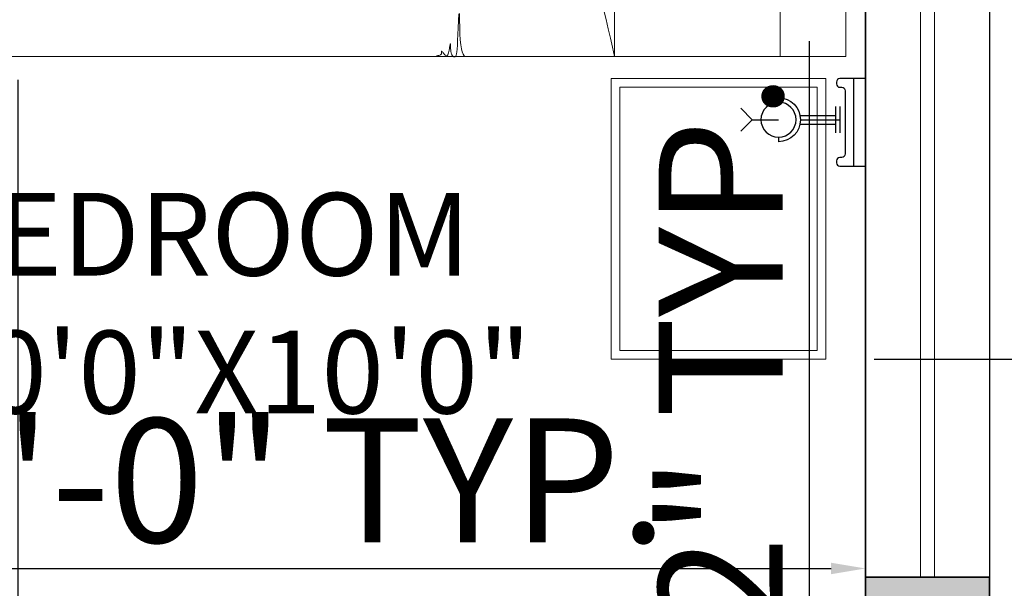
# Model space of a CAD drawing. Units: inches. Extents: x 3321 to 5237, y 11 to 1752.
# Tile 35 of 43: x 5060 to 5131, y 1437 to 1478. Entities that reach past the tile are written whole.
import ezdxf

# ---------------------------------------------------------------- set-up
doc = ezdxf.new("R2010")
doc.units = ezdxf.units.IN
for name, color, linetype, lineweight in [('A-ANNO-DIMS', 2, 'Continuous', 18), ('A-AREA-IDEN', 7, 'Continuous', 18), ('A-COLS', 1, 'Continuous', 35), ('A-FLOR-EDGE', 7, 'Continuous', 25), ('A-GLAZ', 5, 'Continuous', 18), ('A-WALL', 7, 'Continuous', 35), ('FUR', 42, 'Continuous', 18)]:
    doc.layers.add(name, color=color, linetype=linetype, lineweight=lineweight)
for name, color, linetype in [('CEIL', 4, 'Continuous'), ('ELEC', 4, 'Continuous'), ('wood', 26, 'Continuous')]:
    doc.layers.add(name, color=color, linetype=linetype)
doc.styles.get("Standard").update_dxf_attribs({"font": 'arial.ttf'})
doc.dimstyles.new('ISO-25', dxfattribs={"dimtxt": 9, "dimasz": 2.5, "dimexe": 1.25, "dimexo": 0.625, "dimtad": 1, "dimdec": 1, "dimlunit": 3, "dimtxsty": 'Standard', "dimcen": 2.5, "dimclrd": 4, "dimclre": 4, "dimclrt": 256, "dimadec": 0, "dimazin": 0, "dimtfac": 1, "dimtdec": 1, "dimtmove": 0, "dimatfit": 3, "dimfxl": 1, "dimarcsym": 0})

# ---------------------------------------------------------------- blocks, each defined once
blk = doc.blocks.new('BED1')
for p, q in [((0, -1000), (0, 800)), ((150, 800), (0, 800)), ((150, 800), (150, -1000)), ((2058.7, 800), (150, 800)), ((528, 800), (528, -1000))]:
    blk.add_line(p, q)
for points in [[(934, 797.9), (930.9, 797.7), (928.3, 797.4), (926.3, 796.9), (924.9, 796.3), (923.8, 795.6), (923.1, 794.8), (922.7, 793.8), (922.5, 792.7), (922.4, 791.5), (922.5, 790.3), (922.6, 789.2), (922.6, 788.3), (922.6, 787.6), (922.4, 787.3), (922, 787.4), (921.4, 787.9), (920.6, 788.9), (919.5, 790.2), (918.4, 791.6), (917.1, 793.1), (915.9, 794.6), (914.6, 796), (913.3, 797.1), (912.2, 797.9), (911.1, 798.3), (910.1, 798.4), (909.2, 798), (908.3, 797.1), (907.5, 795.8), (906.8, 793.9), (906, 791.4), (905.4, 788.5), (904.8, 785.2), (904.2, 781.7), (903.7, 778.4), (903.2, 775.4), (902.8, 772.9), (902.5, 771.3), (902.3, 770.6), (902.1, 771.2), (902, 772.8), (901.8, 775.2), (901.7, 778.1), (901.5, 781.5), (901.2, 785), (900.8, 788.4), (900.2, 791.5), (899.5, 794.1), (898.6, 796.2), (897.6, 797.9), (896.5, 799.2), (895.3, 800), (894.1, 800.5), (893, 800.7), (891.9, 800.5), (890.9, 800.1), (890, 799), (889.1, 797.1), (888.3, 794), (887.6, 789.3), (886.9, 782.9), (886.2, 774.2), (885.5, 763.1), (884.8, 749.5), (884.2, 734.2), (883.6, 718.3), (883, 702.8)], [(881.2, 701.5), (881.1, 716.8), (880.8, 732.6), (880.2, 748), (879.4, 761.8), (878.3, 773.2), (876.9, 782.2), (875.1, 789.2), (872.9, 794.4), (870.3, 798), (869, 799)]]:
    blk.add_lwpolyline(points)
for centre, radius, start, end in [((3208.8, 1363.3), 2739.4, 191.8679, 206.3247), ((1138.6, 793.9), 983.2, 294.6078, 358.3033)]:
    blk.add_arc(centre, radius, start, end)
blk = doc.blocks.new('APLIQ')
at = {"layer": 'ELEC'}
for p, q in [((0, 0.2), (-0.0261, 0.2261)), ((0, 0.2), (0.0261, 0.2261)), ((0, 0.2), (0, 0.14)), ((-0.05, 0.14), (-0.04, 0.14)), ((0.04, 0.14), (0.05, 0.14)), ((-0.01, 0.09), (-0.01, 0.01)), ((0, 0.09), (0, 0)), ((0.01, 0.09), (0.01, 0.01)), ((-0.03, 0.01), (0.03, 0.01)), ((-0.03, 0), (0.03, 0))]:
    blk.add_line(p, q, dxfattribs=at)
blk.add_circle((0, 0.14), 0.04, dxfattribs=at)
blk.add_arc((0, 0.14), 0.05, 180, 0, dxfattribs=at)
blk = doc.blocks.new('A$C68AE1801')
at = {"layer": 'FUR'}
for points in [[(2.5416, 0), (2.5416, 0.64), (2.0516, 0.64), (2.0516, 0)], [(2.5216, 0.02), (2.5216, 0.62), (2.0716, 0.62), (2.0716, 0.02)]]:
    blk.add_lwpolyline(points, close=True, dxfattribs=at)
at = {"layer": 'wood'}
blk.add_line((2.6057, 0.44), (2.6057, 0.64), dxfattribs=at)
blk.add_lwpolyline([(2.5657, 0.452), (2.5657, 0.448, 0.414214), (2.5737, 0.44), (2.6321, 0.44), (2.6321, 0.64), (2.5737, 0.64, 0.414214), (2.5657, 0.632), (2.5657, 0.628, 0.414214), (2.5737, 0.62), (2.5777, 0.62, -0.414214), (2.5857, 0.612), (2.5857, 0.468, -0.414214), (2.5777, 0.46), (2.5737, 0.46, 0.414214)], format="xyb", close=True, dxfattribs=at)
at = {"layer": 'CEIL', "xscale": -1, "rotation": 90}
blk.add_blockref('APLIQ', (2.5736, 0.546), dxfattribs=at)
at = {"layer": 'FUR', "xscale": 0.001, "yscale": 0.001, "zscale": 0.001, "rotation": 180}
blk.add_blockref('BED1', (2.5872, 1.49), dxfattribs=at)
blk = doc.blocks.new('COL-9X12-FURN-PLAN')
h = blk.add_hatch(color=256)
h.dxf.hatch_style = 1
h.paths.add_polyline_path([(0, 12), (0, 0), (9, 0), (9, 12)])
blk.add_lwpolyline([(0, 0), (9, 0), (9, 12), (0, 12)], close=True)
blk = doc.blocks.new('WIN-48IN-9IN-WALL')
for p, q in [((0, 0), (0, 9)), ((48, 0), (48, 9)), ((0, 5), (48, 5)), ((0, 4), (48, 4))]:
    blk.add_line(p, q)
blk = doc.blocks.new('*D193')
at = {"layer": 'A-ANNO-DIMS', "color": 4, "lineweight": -2, "transparency": 16777216}
for p, q in [((5136.264, 1554.339), (5136.264, 1691.492)), ((5121.709, 1554.339), (5137.514, 1554.339)), ((5136.264, 1455.641), (5136.264, 1551.839)), ((5121.709, 1453.141), (5137.514, 1453.141))]:
    blk.add_line(p, q, dxfattribs=at)
at = {"layer": 'A-ANNO-DIMS', "color": 4, "transparency": 16777216}
for points in [[(5135.847, 1551.839), (5136.68, 1551.839), (5136.264, 1554.339)], [(5135.847, 1455.641), (5136.68, 1455.641), (5136.264, 1453.141)]]:
    blk.add_solid(points, dxfattribs=at)
at = {"layer": 'Defpoints', "color": 0, "transparency": 16777216}
for p in [(5121.084, 1554.339), (5136.264, 1554.339), (5121.084, 1453.141)]:
    blk.add_point(p, dxfattribs=at)
at = {"layer": 'A-ANNO-DIMS', "transparency": 16777216, "insert": (5130.982, 1624.165), "char_height": 9, "attachment_point": 5, "rotation": 90}
blk.add_mtext('BED GROUP 8\'-5" TYP.', dxfattribs=at)
blk = doc.blocks.new('*D194')
at = {"layer": 'A-ANNO-DIMS', "color": 4, "lineweight": -2, "transparency": 16777216}
for p, q in [((5037.321, 1452.516), (5037.321, 1436.712)), ((5121.084, 1452.516), (5121.084, 1436.712)), ((5039.821, 1437.962), (5118.584, 1437.962))]:
    blk.add_line(p, q, dxfattribs=at)
at = {"layer": 'A-ANNO-DIMS', "color": 4, "transparency": 16777216}
for points in [[(5039.821, 1438.379), (5039.821, 1437.545), (5037.321, 1437.962)], [(5118.584, 1438.379), (5118.584, 1437.545), (5121.084, 1437.962)]]:
    blk.add_solid(points, dxfattribs=at)
at = {"layer": 'Defpoints', "color": 0, "transparency": 16777216}
for p in [(5037.321, 1453.141), (5121.084, 1453.141), (5121.084, 1437.962)]:
    blk.add_point(p, dxfattribs=at)
at = {"layer": 'A-ANNO-DIMS', "transparency": 16777216, "insert": (5079.203, 1443.182), "char_height": 9, "attachment_point": 5}
blk.add_mtext('7\'-0" TYP.', dxfattribs=at)
blk = doc.blocks.new('*D197')
at = {"layer": 'A-ANNO-DIMS', "color": 4, "lineweight": -2, "transparency": 16777216}
for p, q in [((5117.009, 1364.83), (5117.009, 1476.212)), ((5114.11, 1364.83), (5118.259, 1364.83)), ((5117.009, 1343.839), (5117.009, 1362.33)), ((5114.11, 1341.339), (5118.259, 1341.339))]:
    blk.add_line(p, q, dxfattribs=at)
at = {"layer": 'A-ANNO-DIMS', "color": 4, "transparency": 16777216}
for points in [[(5116.592, 1362.33), (5117.426, 1362.33), (5117.009, 1364.83)], [(5116.592, 1343.839), (5117.426, 1343.839), (5117.009, 1341.339)]]:
    blk.add_solid(points, dxfattribs=at)
at = {"layer": 'Defpoints', "color": 0, "transparency": 16777216}
for p in [(5113.485, 1364.83), (5117.009, 1364.83), (5113.485, 1341.339)]:
    blk.add_point(p, dxfattribs=at)
at = {"layer": 'A-ANNO-DIMS', "transparency": 16777216, "insert": (5111.731, 1421.771), "char_height": 9, "attachment_point": 5, "rotation": 90}
blk.add_mtext('WC 1\'-11 1/2" TYP.', dxfattribs=at)
blk = doc.blocks.new('*D199')
at = {"layer": 'A-ANNO-DIMS', "color": 4, "lineweight": -2, "transparency": 16777216}
for p, q in [((5059.569, 1379.636), (5059.569, 1473.411)), ((5060.444, 1379.636), (5058.319, 1379.636)), ((5059.569, 1372.136), (5059.569, 1377.136)), ((5060.444, 1369.636), (5058.319, 1369.636))]:
    blk.add_line(p, q, dxfattribs=at)
at = {"layer": 'A-ANNO-DIMS', "color": 4, "transparency": 16777216}
for points in [[(5059.153, 1377.136), (5059.986, 1377.136), (5059.569, 1379.636)], [(5059.153, 1372.136), (5059.986, 1372.136), (5059.569, 1369.636)]]:
    blk.add_solid(points, dxfattribs=at)
at = {"layer": 'Defpoints', "color": 0, "transparency": 16777216}
for p in [(5059.569, 1379.636), (5061.069, 1379.636), (5061.069, 1369.636)]:
    blk.add_point(p, dxfattribs=at)
at = {"layer": 'A-ANNO-DIMS', "transparency": 16777216, "insert": (5054.349, 1427.773), "char_height": 9, "attachment_point": 5, "rotation": 90}
blk.add_mtext('TAP 0\'-10" TYP.', dxfattribs=at)

msp = doc.modelspace()

# ---------------------------------------------------------------- linework, layer by layer
at = {"layer": 'A-FLOR-EDGE'}
msp.add_line((5130.084, 1687.339), (5130.084, 1091.339), dxfattribs=at)
at = {"layer": 'A-WALL'}
msp.add_line((5121.084, 1554.339), (5121.084, 1434.339), dxfattribs=at)

# ---------------------------------------------------------------- block references
at = {"layer": 'A-COLS'}
msp.add_blockref('COL-9X12-FURN-PLAN', (5121.084, 1425.339), dxfattribs=at)
at = {"layer": 'A-GLAZ', "rotation": 90.00000000000043}
msp.add_blockref('WIN-48IN-9IN-WALL', (5130.084, 1437.339), dxfattribs=at)
at = {"layer": 'FUR', "xscale": 31.82298296329056, "yscale": 31.82298296329056, "zscale": 31.82298296329056}
msp.add_blockref('A$C68AE1801', (5037.321, 1453.141), dxfattribs=at)

# ---------------------------------------------------------------- texts
at = {"layer": 'A-AREA-IDEN', "insert": (5052.569, 1465.211), "char_height": 6, "attachment_point": 1}
msp.add_mtext_dynamic_manual_height_columns('BEDROOM\\P10\'0"X10\'0"', width=97.3114, gutter_width=25, heights=[0], dxfattribs=at)

# ---------------------------------------------------------------- dimensions: what is measured, and where the dimension line sits
at = {"layer": 'A-ANNO-DIMS'}
for base, p1, p2, text, picture, middle in [((5136.264, 1554.339), (5121.084, 1453.141), (5121.084, 1554.339), 'BED GROUP <> TYP.', '*D193', (5130.982, 1624.165)), ((5117.009, 1364.83), (5113.485, 1341.339), (5113.485, 1364.83), 'WC <> TYP.', '*D197', (5111.731, 1421.771)), ((5059.569, 1379.636), (5061.069, 1369.636), (5061.069, 1379.636), 'TAP <> TYP.', '*D199', (5054.349, 1427.773))]:
    dim = msp.add_linear_dim(base=base, p1=p1, p2=p2, angle=90, text=text, dimstyle='ISO-25', override={"dimdec": 1, "dimlfac": 1, "dimrnd": 0, "dimzin": 1, "dimdsep": 46, "dimlunit": 4, "dimfrac": 2}, dxfattribs=at)
    dim.commit()
    dim.dimension.update_dxf_attribs({"geometry": picture, "text_midpoint": middle})
dim = msp.add_linear_dim(base=(5121.084, 1437.962), p1=(5037.321, 1453.141), p2=(5121.084, 1453.141), text='<> TYP.', dimstyle='ISO-25', override={"dimdec": 1, "dimlfac": 1, "dimrnd": 0, "dimzin": 1, "dimdsep": 46, "dimlunit": 4, "dimfrac": 2}, dxfattribs=at)
dim.commit()
dim.dimension.update_dxf_attribs({"geometry": '*D194', "text_midpoint": (5079.203, 1443.182)})

doc.saveas('drawing.dxf')
